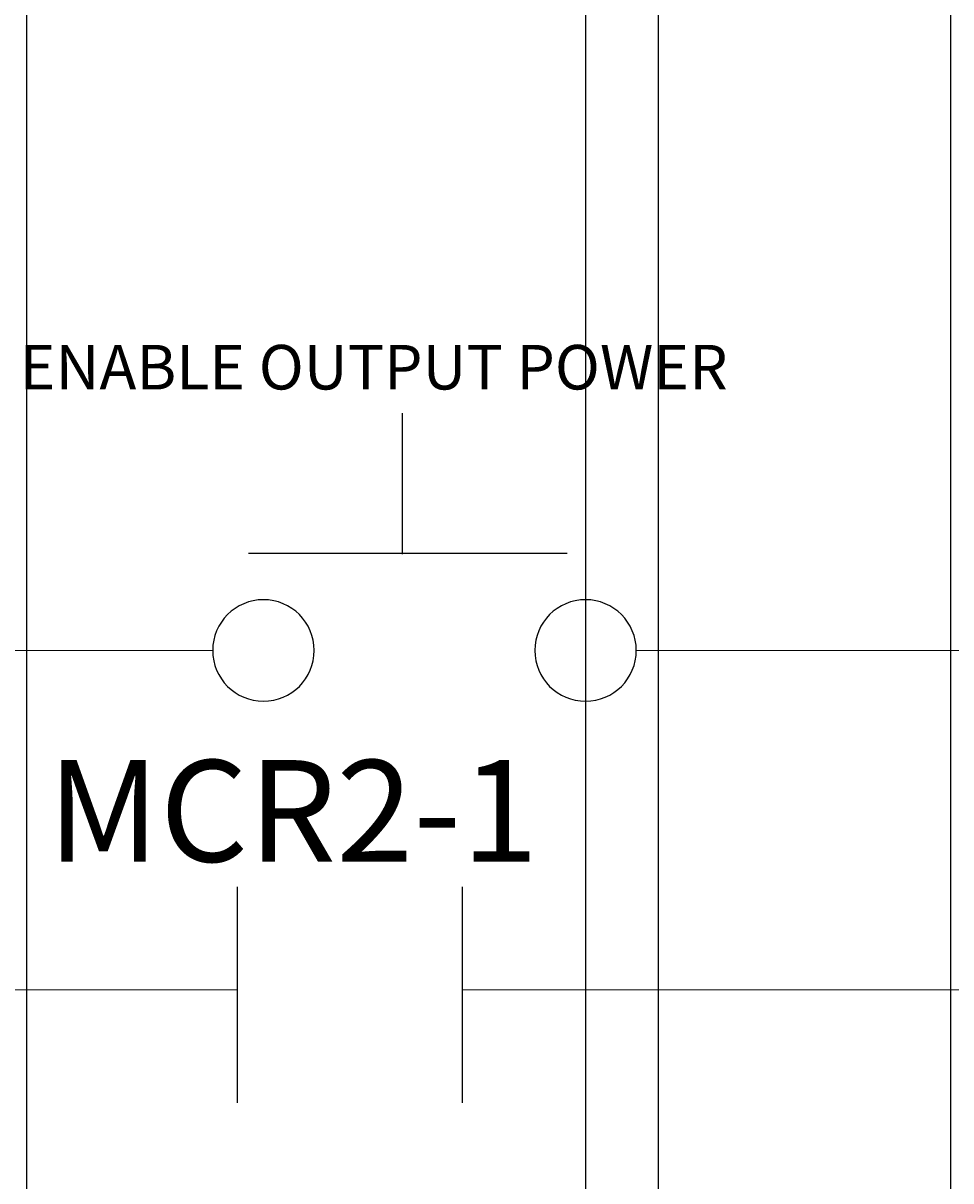
# Model space of a CAD drawing. Units: inches. Extents: x 738 to 1068, y 378 to 757.
# Tile 17 of 41: x 856 to 901, y 435 to 492. Entities that reach past the tile are written whole.
import ezdxf

# ---------------------------------------------------------------- set-up
doc = ezdxf.new("R2010")
doc.units = ezdxf.units.IN
doc.header["$MEASUREMENT"] = 0
for name, color, linetype, lineweight in [('A-ANNO-DIMS', 2, 'Continuous', 18), ('E-ANNO-TEXT', 7, 'Continuous', 18), ('E-CTRL-CONT', 4, 'Continuous', 25), ('E-CTRL-PBTN', 4, 'Continuous', 25), ('E-CTRL-WIRE', 7, 'Continuous', 18)]:
    doc.layers.add(name, color=color, linetype=linetype, lineweight=lineweight)
doc.styles.get("Standard").update_dxf_attribs({"font": 'arial.ttf'})
doc.dimstyles.get("Standard").update_dxf_attribs({"dimtxt": 0.18, "dimasz": 0.18, "dimexe": 0.18, "dimexo": 0.0625, "dimgap": 0.09, "dimtad": 0, "dimtih": 1, "dimtoh": 1, "dimdec": 4, "dimzin": 0, "dimdsep": 46, "dimtxsty": 'Standard', "dimcen": 0.09, "dimadec": 0, "dimazin": 0, "dimtfac": 1, "dimtdec": 4, "dimtofl": 0, "dimtmove": 0, "dimatfit": 3, "dimfxl": 1, "dimtolj": 1, "dimtzin": 0, "dimarcsym": 0})

# ---------------------------------------------------------------- blocks, each defined once
blk = doc.blocks.new('PB-ENABLE-NO')
for p, q in [((9.342, 7.241), (9.342, 14.19)), ((1.764, 7.299), (17.45, 7.299))]:
    blk.add_line(p, q)
for points in [[(0, 2.5, 1), (5, 2.5, 1)], [(15.861, 2.5, 1), (20.861, 2.5, 1)]]:
    blk.add_lwpolyline(points, format="xyb", close=True)
blk = doc.blocks.new('MCR-HOLD-CONTACT-NO')
for p, q in [((0, 0), (0, 10.627)), ((11.061, 10.627), (11.061, 0))]:
    blk.add_line(p, q)
blk = doc.blocks.new('*D27')
at = {"layer": 'A-ANNO-DIMS', "color": 0, "lineweight": -2, "transparency": 16777216}
for p, q in [((883.457, 646.923), (883.457, 378.239)), ((923.511, 646.923), (923.511, 378.239)), ((883.637, 378.419), (903.086, 378.419)), ((923.331, 378.419), (903.882, 378.419))]:
    blk.add_line(p, q, dxfattribs=at)
at = {"layer": 'A-ANNO-DIMS', "color": 0, "transparency": 16777216}
for points in [[(883.637, 378.449), (883.637, 378.389), (883.457, 378.419)], [(923.331, 378.449), (923.331, 378.389), (923.511, 378.419)]]:
    blk.add_solid(points, dxfattribs=at)
at = {"layer": 'Defpoints', "color": 0, "transparency": 16777216}
for p in [(883.457, 646.985), (923.511, 646.985), (923.511, 378.419)]:
    blk.add_point(p, dxfattribs=at)
at = {"layer": 'A-ANNO-DIMS', "color": 0, "transparency": 16777216, "insert": (903.484, 378.419), "char_height": 0.18, "attachment_point": 5}
blk.add_mtext('\\A1;40.05', dxfattribs=at)
blk = doc.blocks.new('*D33')
at = {"layer": 'A-ANNO-DIMS', "color": 0, "lineweight": -2, "transparency": 16777216}
for p, q in [((836.324, 514.624), (836.324, 378.239)), ((907.171, 514.624), (907.171, 378.239)), ((836.504, 378.419), (871.354, 378.419)), ((906.991, 378.419), (872.141, 378.419))]:
    blk.add_line(p, q, dxfattribs=at)
at = {"layer": 'A-ANNO-DIMS', "color": 0, "transparency": 16777216}
for points in [[(836.504, 378.449), (836.504, 378.389), (836.324, 378.419)], [(906.991, 378.449), (906.991, 378.389), (907.171, 378.419)]]:
    blk.add_solid(points, dxfattribs=at)
at = {"layer": 'Defpoints', "color": 0, "transparency": 16777216}
for p in [(836.324, 514.687), (907.171, 514.687), (907.171, 378.419)]:
    blk.add_point(p, dxfattribs=at)
at = {"layer": 'A-ANNO-DIMS', "color": 0, "transparency": 16777216, "insert": (871.748, 378.419), "char_height": 0.18, "attachment_point": 5}
blk.add_mtext('\\A1;70.85', dxfattribs=at)
blk = doc.blocks.new('*D35')
at = {"layer": 'A-ANNO-DIMS', "color": 0, "lineweight": -2, "transparency": 16777216}
for p, q in [((855.932, 686.266), (855.932, 378.239)), ((901.429, 686.267), (901.429, 378.239)), ((856.112, 378.419), (878.352, 378.419)), ((901.249, 378.419), (879.009, 378.419))]:
    blk.add_line(p, q, dxfattribs=at)
at = {"layer": 'A-ANNO-DIMS', "color": 0, "transparency": 16777216}
for points in [[(856.112, 378.449), (856.112, 378.389), (855.932, 378.419)], [(901.249, 378.449), (901.249, 378.389), (901.429, 378.419)]]:
    blk.add_solid(points, dxfattribs=at)
at = {"layer": 'Defpoints', "color": 0, "transparency": 16777216}
for p in [(855.932, 686.329), (901.429, 686.329), (901.429, 378.419)]:
    blk.add_point(p, dxfattribs=at)
at = {"layer": 'A-ANNO-DIMS', "color": 0, "transparency": 16777216, "insert": (878.68, 378.419), "char_height": 0.18, "attachment_point": 5}
blk.add_mtext('\\A1;45.5', dxfattribs=at)
blk = doc.blocks.new('*D38')
at = {"layer": 'A-ANNO-DIMS', "color": 0, "lineweight": -2, "transparency": 16777216}
for p, q in [((781.485, 593.017), (781.485, 378.239)), ((887.04, 593.067), (887.04, 378.239)), ((781.665, 378.419), (833.807, 378.419)), ((886.86, 378.419), (834.718, 378.419))]:
    blk.add_line(p, q, dxfattribs=at)
at = {"layer": 'A-ANNO-DIMS', "color": 0, "transparency": 16777216}
for points in [[(781.665, 378.449), (781.665, 378.389), (781.485, 378.419)], [(886.86, 378.449), (886.86, 378.389), (887.04, 378.419)]]:
    blk.add_solid(points, dxfattribs=at)
at = {"layer": 'Defpoints', "color": 0, "transparency": 16777216}
for p in [(781.485, 593.08), (887.04, 593.13), (887.04, 378.419)]:
    blk.add_point(p, dxfattribs=at)
at = {"layer": 'A-ANNO-DIMS', "color": 0, "transparency": 16777216, "insert": (834.263, 378.419), "char_height": 0.18, "attachment_point": 5}
blk.add_mtext('\\A1;105.56', dxfattribs=at)
blk = doc.blocks.new('*D39')
at = {"layer": 'A-ANNO-DIMS', "color": 0, "lineweight": -2, "transparency": 16777216}
for p, q in [((887.04, 581.418), (887.04, 378.239)), ((938.455, 581.418), (938.455, 378.239)), ((887.22, 378.419), (912.371, 378.419)), ((938.275, 378.419), (913.124, 378.419))]:
    blk.add_line(p, q, dxfattribs=at)
at = {"layer": 'A-ANNO-DIMS', "color": 0, "transparency": 16777216}
for points in [[(887.22, 378.449), (887.22, 378.389), (887.04, 378.419)], [(938.275, 378.449), (938.275, 378.389), (938.455, 378.419)]]:
    blk.add_solid(points, dxfattribs=at)
at = {"layer": 'Defpoints', "color": 0, "transparency": 16777216}
for p in [(887.04, 581.481), (938.455, 581.481), (938.455, 378.419)]:
    blk.add_point(p, dxfattribs=at)
at = {"layer": 'A-ANNO-DIMS', "color": 0, "transparency": 16777216, "insert": (912.748, 378.419), "char_height": 0.18, "attachment_point": 5}
blk.add_mtext('\\A1;51.41', dxfattribs=at)

msp = doc.modelspace()

# ---------------------------------------------------------------- linework, layer by layer
at = {"layer": 'E-CTRL-WIRE'}
for p, q in [((809.3803, 461.3919), (865.0964, 461.3919)), ((885.9574, 461.3919), (966.9395, 461.3919)), ((866.3244, 444.6775), (836.3244, 444.6775)), ((877.3586, 444.6775), (907.3586, 444.6775))]:
    msp.add_line(p, q, dxfattribs=at)

# ---------------------------------------------------------------- block references
at = {"layer": 'E-CTRL-CONT'}
msp.add_blockref('MCR-HOLD-CONTACT-NO', (866.324, 439.116), dxfattribs=at)
at = {"layer": 'E-CTRL-PBTN'}
msp.add_blockref('PB-ENABLE-NO', (865.096, 458.892), dxfattribs=at)

# ---------------------------------------------------------------- texts
at = {"layer": 'E-ANNO-TEXT'}
for s, height, p in [('ENABLE OUTPUT POWER', 2.19392, (855.593, 474.2478)), ('MCR2-1', 5.00518, (856.9472, 450.9853))]:
    msp.add_text(s, height=height, dxfattribs=at).set_placement(p)

# ---------------------------------------------------------------- dimensions: what is measured, and where the dimension line sits
at = {"layer": 'A-ANNO-DIMS'}
for base, p1, p2, override, picture, middle in [((901.4286, 378.4191), (855.9323, 686.329), (901.4286, 686.3292), {"dimdec": 1, "dimlfac": 1, "dimrnd": 0, "dimzin": 0, "dimdsep": 46, "dimlunit": 2}, '*D35', (878.6804, 378.4191)), ((923.5105, 378.4191), (883.4574, 646.9853), (923.5105, 646.9853), {"dimdec": 2, "dimlfac": 1, "dimrnd": 0, "dimzin": 0, "dimdsep": 46, "dimlunit": 2}, '*D27', (903.484, 378.4191)), ((887.0404, 378.4191), (781.4846, 593.0796), (887.0404, 593.1296), {"dimdec": 2, "dimlfac": 1, "dimrnd": 0, "dimzin": 0, "dimdsep": 46, "dimlunit": 2}, '*D38', (834.2625, 378.4191)), ((938.455, 378.4191), (887.0404, 581.4808), (938.455, 581.4808), {"dimdec": 2, "dimlfac": 1, "dimrnd": 0, "dimzin": 0, "dimdsep": 46, "dimlunit": 2}, '*D39', (912.7477, 378.4191)), ((907.1708, 378.4191), (836.3244, 514.6866), (907.1708, 514.6866), {"dimdec": 2, "dimlfac": 1, "dimrnd": 0, "dimzin": 0, "dimdsep": 46, "dimlunit": 2}, '*D33', (871.7476, 378.4191))]:
    dim = msp.add_linear_dim(base=base, p1=p1, p2=p2, dimstyle='Standard', override=override, dxfattribs=at)
    dim.commit()
    dim.dimension.update_dxf_attribs({"geometry": picture, "text_midpoint": middle})

doc.saveas('drawing.dxf')
